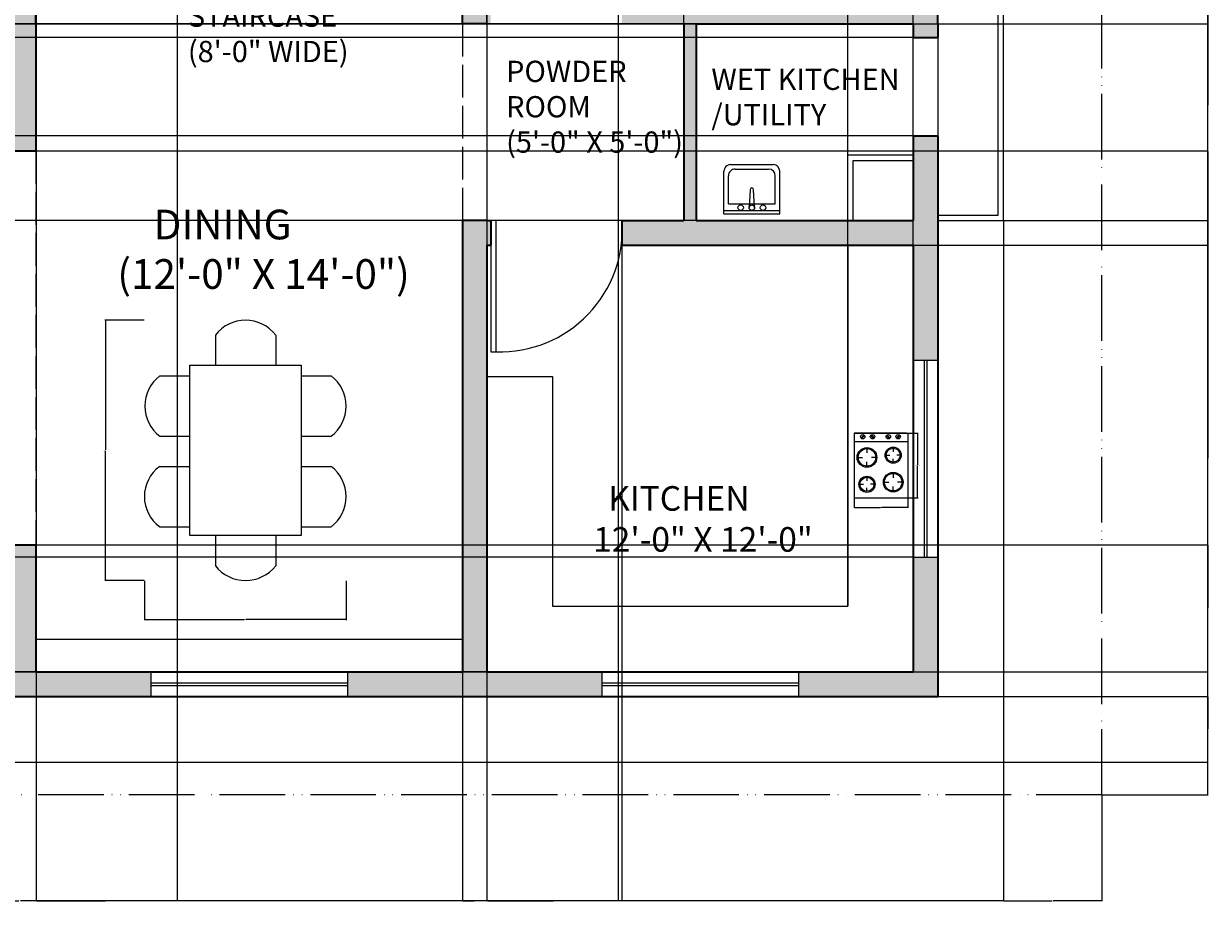
# Model space of a CAD drawing. Units: inches. Extents: x 2847 to 3693, y 1516 to 2098.
# Tile 5 of 6: x 3259 to 3693, y 1516 to 1837. Entities that reach past the tile are written whole.
import ezdxf

# ---------------------------------------------------------------- set-up
doc = ezdxf.new("R2010")
doc.units = ezdxf.units.IN
doc.linetypes.add('ACAD_ISO02W100', pattern=[15, 12, -3])
doc.linetypes.add('ACAD_ISO05W100', pattern=[33, 24, -3, 0, -3, 0, -3])
for name, color, linetype, lineweight in [('A-ANNO-DIMS', 2, 'Continuous', 18), ('A-AREA-IDEN', 7, 'Continuous', 18), ('A-DOOR', 3, 'Continuous', 18), ('A-EQPM', 9, 'Continuous', 18), ('A-FLOR', 7, 'Continuous', 25), ('A-FLOR-CASE', 8, 'Continuous', 18), ('A-FLOR-FIXT', 9, 'Continuous', 18), ('A-FLOR-OVHD', 8, 'ACAD_ISO02W100', 13), ('A-FURN', 8, 'Continuous', 18), ('A-GLAZ', 4, 'Continuous', 18), ('A-WALL', 7, 'Continuous', 35), ('C-PROP', 7, 'ACAD_ISO05W100', 18)]:
    doc.layers.add(name, color=color, linetype=linetype, lineweight=lineweight)
doc.layers.add('A-WALL-PATT', color=251, linetype='Continuous', lineweight=13, true_color=0x636466)
doc.styles.get("Standard").update_dxf_attribs({"font": 'arial.ttf'})
doc.dimstyles.get("Standard").update_dxf_attribs({"dimtxt": 0.18, "dimasz": 0.18, "dimexe": 0.18, "dimexo": 0.0625, "dimgap": 0.09, "dimtad": 0, "dimtih": 1, "dimtoh": 1, "dimdec": 4, "dimzin": 0, "dimdsep": 46, "dimtxsty": 'Standard', "dimcen": 0.09, "dimadec": 0, "dimazin": 0, "dimtfac": 1, "dimtdec": 4, "dimtofl": 0, "dimtmove": 0, "dimatfit": 3, "dimfxl": 1, "dimtolj": 1, "dimtzin": 0, "dimarcsym": 0})

# ---------------------------------------------------------------- blocks, each defined once
blk = doc.blocks.new('DINING TABLE')
for p, q in [((2443.51, 1632.65), (2443.51, 1644.65)), ((2467.51, 1632.65), (2467.51, 1644.65)), ((2479.51, 1632.65), (2479.51, 1644.65)), ((2503.51, 1632.65), (2503.51, 1644.65)), ((2427.28, 1622.52), (2439.28, 1622.52)), ((2507.03, 1622.52), (2519.03, 1622.52)), ((2427.28, 1598.52), (2439.28, 1598.52)), ((2507.03, 1598.52), (2519.03, 1598.52)), ((2443.51, 1576.39), (2443.51, 1588.39)), ((2467.51, 1576.39), (2467.51, 1588.39)), ((2479.51, 1576.39), (2479.51, 1588.39)), ((2503.51, 1576.39), (2503.51, 1588.39))]:
    blk.add_line(p, q)
blk.add_lwpolyline([(2439.28, 1632.65), (2507.03, 1632.65), (2507.03, 1588.39), (2439.28, 1588.39)], close=True)
for centre, radius, start, end in [((2455.51, 1635.3), 15.21, 37.9308, 142.0692), ((2491.51, 1635.3), 15.21, 37.9308, 142.0692), ((2436.64, 1610.52), 15.21, 127.9308, 232.0692), ((2509.67, 1610.52), 15.21, 307.9308, 52.0692), ((2455.51, 1585.74), 15.21, 217.9308, 322.0692), ((2491.51, 1585.15), 14.86, 216.1262, 323.8738)]:
    blk.add_arc(centre, radius, start, end)
blk = doc.blocks.new('A$C16A60262')
at = {"linetype": 'ByBlock'}
for p, q in [((0, 600), (0, 0)), ((488, 600), (0, 600)), ((0, 600), (500, 600)), ((0, 600), (500, 600)), ((500, 600), (500, 0)), ((500, 600), (500, 0)), ((500, 520), (0, 520)), ((119, 456), (119, 415)), ((363, 460), (363, 427)), ((38, 374), (79, 374)), ((119, 293), (119, 334)), ((201, 374), (160, 374)), ((298, 395), (331, 395)), ((363, 330), (363, 362)), ((428, 395), (396, 395)), ((363, 225), (363, 185)), ((54, 124), (87, 124)), ((119, 189), (119, 156)), ((184, 124), (152, 124)), ((282, 144), (323, 144)), ((445, 144), (404, 144)), ((0, 0), (500, 0)), ((119, 59), (119, 91)), ((363, 63), (363, 103))]:
    blk.add_line(p, q, dxfattribs=at)
for p, q in [((66, 557), (87, 579)), ((72, 552), (66, 557)), ((93, 573), (72, 552)), ((87, 579), (93, 573)), ((158, 572), (163, 578)), ((179, 551), (158, 572)), ((163, 578), (184, 557)), ((184, 557), (179, 551)), ((305, 572), (311, 578)), ((326, 551), (305, 572)), ((311, 578), (332, 557)), ((332, 557), (326, 551)), ((396, 558), (417, 580)), ((402, 553), (396, 558)), ((423, 574), (402, 553)), ((417, 580), (423, 574))]:
    blk.add_line(p, q)
for centre in [(80, 566), (171, 566), (318, 566), (409, 566)]:
    blk.add_circle(centre, 20.6)
for centre, radius in [((119, 374), 91.3), ((119, 374), 81.3), ((363, 395), 75), ((363, 395), 65), ((363, 144), 91.3), ((363, 144), 81.3), ((119, 124), 75), ((119, 124), 65)]:
    blk.add_circle(centre, radius, dxfattribs=at)
blk = doc.blocks.new('A$C5C4020F2')
for p, q in [((0.5, 0.44), (0, 0.44)), ((0, 0.44), (0, 0.06)), ((0.5, 0.44), (0.5, 0.06)), ((0.5, 0.41), (0, 0.41)), ((0.04, 0.35), (0.04, 0.1)), ((0.46, 0.35), (0.04, 0.35)), ((0.225, 0.384), (0.234, 0.224)), ((0.266, 0.224), (0.275, 0.384)), ((0.46, 0.35), (0.46, 0.1)), ((0.4, 0.04), (0.1, 0.04)), ((0.44, 0), (0.06, 0))]:
    blk.add_line(p, q)
for centre in [(0.15, 0.385), (0.25, 0.385), (0.35, 0.385)]:
    blk.add_circle(centre, 0.025)
for centre, radius, start, end in [((0.25, 0.225), 0.016, 183.2169, 356.7831), ((0.06, 0.06), 0.06, 180, 270), ((0.1, 0.1), 0.06, 180, 270), ((0.4, 0.1), 0.06, 270, 0), ((0.44, 0.06), 0.06, 270, 0)]:
    blk.add_arc(centre, radius, start, end)
blk = doc.blocks.new('WIN-GLAZ-72IN')
for p, q in [((0, 1), (72, 1)), ((0, 0), (72, 0))]:
    blk.add_line(p, q)
blk = doc.blocks.new('*D27')
at = {"layer": 'A-ANNO-DIMS', "color": 0, "lineweight": -2, "transparency": 16777216}
for p, q in [((3303.45, 1728.67), (3289.06, 1728.67)), ((3289.24, 1728.49), (3289.24, 1681.27)), ((3289.24, 1633.69), (3289.24, 1680.91)), ((3303.45, 1633.51), (3289.06, 1633.51))]:
    blk.add_line(p, q, dxfattribs=at)
at = {"layer": 'A-ANNO-DIMS', "color": 0, "transparency": 16777216}
for points in [[(3289.21, 1728.49), (3289.27, 1728.49), (3289.24, 1728.67)], [(3289.21, 1633.69), (3289.27, 1633.69), (3289.24, 1633.51)]]:
    blk.add_solid(points, dxfattribs=at)
at = {"layer": 'Defpoints', "color": 0, "transparency": 16777216}
for p in [(3303.51, 1728.67), (3289.24, 1633.51), (3303.51, 1633.51)]:
    blk.add_point(p, dxfattribs=at)
at = {"layer": 'A-ANNO-DIMS', "color": 0, "transparency": 16777216, "insert": (3289.24, 1681.09), "char_height": 0.18, "attachment_point": 5}
blk.add_mtext('\\A1;DINING SET 95', dxfattribs=at)
blk = doc.blocks.new('*D28')
at = {"layer": 'A-ANNO-DIMS', "color": 0, "lineweight": -2, "transparency": 16777216}
for p, q in [((3303.51, 1633.45), (3303.51, 1619.05)), ((3377.29, 1633.45), (3377.29, 1619.05)), ((3303.69, 1619.23), (3340.18, 1619.23)), ((3377.11, 1619.23), (3340.62, 1619.23))]:
    blk.add_line(p, q, dxfattribs=at)
at = {"layer": 'A-ANNO-DIMS', "color": 0, "transparency": 16777216}
for points in [[(3303.69, 1619.26), (3303.69, 1619.2), (3303.51, 1619.23)], [(3377.11, 1619.26), (3377.11, 1619.2), (3377.29, 1619.23)]]:
    blk.add_solid(points, dxfattribs=at)
at = {"layer": 'Defpoints', "color": 0, "transparency": 16777216}
for p in [(3303.51, 1633.51), (3377.29, 1633.51), (3377.29, 1619.23)]:
    blk.add_point(p, dxfattribs=at)
at = {"layer": 'A-ANNO-DIMS', "color": 0, "transparency": 16777216, "insert": (3340.4, 1619.23), "char_height": 0.18, "attachment_point": 5}
blk.add_mtext('\\A1;74', dxfattribs=at)
blk = doc.blocks.new('*D29')
at = {"layer": 'A-ANNO-DIMS', "color": 0, "lineweight": -2, "transparency": 16777216}
for p, q in [((3582.95, 1687.44), (3586.61, 1687.44)), ((3586.43, 1687.26), (3586.43, 1675.81)), ((3586.43, 1663.99), (3586.43, 1675.44)), ((3582.95, 1663.81), (3586.61, 1663.81))]:
    blk.add_line(p, q, dxfattribs=at)
at = {"layer": 'A-ANNO-DIMS', "color": 0, "transparency": 16777216}
for points in [[(3586.4, 1687.26), (3586.46, 1687.26), (3586.43, 1687.44)], [(3586.4, 1663.99), (3586.46, 1663.99), (3586.43, 1663.81)]]:
    blk.add_solid(points, dxfattribs=at)
at = {"layer": 'Defpoints', "color": 0, "transparency": 16777216}
for p in [(3582.89, 1687.44), (3586.43, 1687.44), (3582.89, 1663.81)]:
    blk.add_point(p, dxfattribs=at)
at = {"layer": 'A-ANNO-DIMS', "color": 0, "transparency": 16777216, "insert": (3586.43, 1675.63), "char_height": 0.18, "attachment_point": 5}
blk.add_mtext('\\A1;COOKTOP 24', dxfattribs=at)
blk = doc.blocks.new('*D30')
at = {"layer": 'A-ANNO-DIMS', "color": 0, "lineweight": -2, "transparency": 16777216}
for p, q in [((3563.2, 1663.75), (3563.2, 1660.09)), ((3563.38, 1660.27), (3572.82, 1660.27)), ((3582.71, 1660.27), (3573.26, 1660.27)), ((3582.89, 1663.75), (3582.89, 1660.09))]:
    blk.add_line(p, q, dxfattribs=at)
at = {"layer": 'A-ANNO-DIMS', "color": 0, "transparency": 16777216}
for points in [[(3563.38, 1660.3), (3563.38, 1660.24), (3563.2, 1660.27)], [(3582.71, 1660.3), (3582.71, 1660.24), (3582.89, 1660.27)]]:
    blk.add_solid(points, dxfattribs=at)
at = {"layer": 'Defpoints', "color": 0, "transparency": 16777216}
for p in [(3563.2, 1663.81), (3582.89, 1663.81), (3582.89, 1660.27)]:
    blk.add_point(p, dxfattribs=at)
at = {"layer": 'A-ANNO-DIMS', "color": 0, "transparency": 16777216, "insert": (3573.04, 1660.27), "char_height": 0.18, "attachment_point": 5}
blk.add_mtext('\\A1;20', dxfattribs=at)
blk = doc.blocks.new('*D36')
at = {"layer": 'A-ANNO-DIMS', "color": 0, "lineweight": -2, "transparency": 16777216}
for p, q in [((3653.91, 2059.12), (3692.73, 2059.12)), ((3692.55, 2058.94), (3692.55, 1807.3)), ((3692.55, 1555.3), (3692.55, 1806.94)), ((3653.91, 1555.12), (3692.73, 1555.12))]:
    blk.add_line(p, q, dxfattribs=at)
at = {"layer": 'A-ANNO-DIMS', "color": 0, "transparency": 16777216}
for points in [[(3692.52, 2058.94), (3692.58, 2058.94), (3692.55, 2059.12)], [(3692.52, 1555.3), (3692.58, 1555.3), (3692.55, 1555.12)]]:
    blk.add_solid(points, dxfattribs=at)
at = {"layer": 'Defpoints', "color": 0, "transparency": 16777216}
for p in [(3653.85, 2059.12), (3692.55, 2059.12), (3653.85, 1555.12)]:
    blk.add_point(p, dxfattribs=at)
at = {"layer": 'A-ANNO-DIMS', "color": 0, "transparency": 16777216, "insert": (3692.55, 1807.12), "char_height": 0.18, "attachment_point": 5}
blk.add_mtext('\\A1;504', dxfattribs=at)
blk = doc.blocks.new('*D37')
at = {"layer": 'A-ANNO-DIMS', "color": 0, "lineweight": -2, "transparency": 16777216}
for p, q in [((3617.85, 1765.06), (3617.85, 1516.24)), ((2897.85, 1591.06), (2897.85, 1516.24)), ((2898.03, 1516.42), (3257.56, 1516.42)), ((3617.67, 1516.42), (3258.13, 1516.42))]:
    blk.add_line(p, q, dxfattribs=at)
at = {"layer": 'A-ANNO-DIMS', "color": 0, "transparency": 16777216}
for points in [[(2898.03, 1516.45), (2898.03, 1516.39), (2897.85, 1516.42)], [(3617.67, 1516.45), (3617.67, 1516.39), (3617.85, 1516.42)]]:
    blk.add_solid(points, dxfattribs=at)
at = {"layer": 'Defpoints', "color": 0, "transparency": 16777216}
for p in [(3617.85, 1765.12), (2897.85, 1591.12), (3617.85, 1516.42)]:
    blk.add_point(p, dxfattribs=at)
at = {"layer": 'A-ANNO-DIMS', "color": 0, "transparency": 16777216, "insert": (3257.85, 1516.42), "char_height": 0.18, "attachment_point": 5}
blk.add_mtext('\\A1;720', dxfattribs=at)
blk = doc.blocks.new('*D46')
at = {"layer": 'A-ANNO-DIMS', "color": 0, "lineweight": -2, "transparency": 16777216}
for p, q in [((3584.91, 1756.12), (3692.73, 1756.12)), ((3692.55, 1755.94), (3692.55, 1678.3)), ((3692.55, 1600.3), (3692.55, 1677.94)), ((3584.91, 1600.12), (3692.73, 1600.12))]:
    blk.add_line(p, q, dxfattribs=at)
at = {"layer": 'A-ANNO-DIMS', "color": 0, "transparency": 16777216}
for points in [[(3692.52, 1755.94), (3692.58, 1755.94), (3692.55, 1756.12)], [(3692.52, 1600.3), (3692.58, 1600.3), (3692.55, 1600.12)]]:
    blk.add_solid(points, dxfattribs=at)
at = {"layer": 'Defpoints', "color": 0, "transparency": 16777216}
for p in [(3584.85, 1756.12), (3692.55, 1756.12), (3584.85, 1600.12)]:
    blk.add_point(p, dxfattribs=at)
at = {"layer": 'A-ANNO-DIMS', "color": 0, "transparency": 16777216, "insert": (3692.55, 1678.12), "char_height": 0.18, "attachment_point": 5}
blk.add_mtext('\\A1;156', dxfattribs=at)
blk = doc.blocks.new('*D47')
at = {"layer": 'A-ANNO-DIMS', "color": 0, "lineweight": -2, "transparency": 16777216}
for p, q in [((3617.91, 1960.12), (3692.73, 1960.12)), ((3692.55, 1959.94), (3692.55, 1862.8)), ((3692.55, 1765.3), (3692.55, 1862.44)), ((3617.91, 1765.12), (3692.73, 1765.12))]:
    blk.add_line(p, q, dxfattribs=at)
at = {"layer": 'A-ANNO-DIMS', "color": 0, "transparency": 16777216}
for points in [[(3692.52, 1959.94), (3692.58, 1959.94), (3692.55, 1960.12)], [(3692.52, 1765.3), (3692.58, 1765.3), (3692.55, 1765.12)]]:
    blk.add_solid(points, dxfattribs=at)
at = {"layer": 'Defpoints', "color": 0, "transparency": 16777216}
for p in [(3617.85, 1960.12), (3692.55, 1960.12), (3617.85, 1765.12)]:
    blk.add_point(p, dxfattribs=at)
at = {"layer": 'A-ANNO-DIMS', "color": 0, "transparency": 16777216, "insert": (3692.55, 1862.62), "char_height": 0.18, "attachment_point": 5}
blk.add_mtext('\\A1;195', dxfattribs=at)
blk = doc.blocks.new('*D50')
at = {"layer": 'A-ANNO-DIMS', "color": 0, "lineweight": -2, "transparency": 16777216}
for p, q in [((2989.41, 2011.12), (3692.73, 2011.12)), ((3692.55, 2010.94), (3692.55, 1924.3)), ((3692.55, 1837.3), (3692.55, 1923.94)), ((2989.41, 1837.12), (3692.73, 1837.12))]:
    blk.add_line(p, q, dxfattribs=at)
at = {"layer": 'A-ANNO-DIMS', "color": 0, "transparency": 16777216}
for points in [[(3692.52, 2010.94), (3692.58, 2010.94), (3692.55, 2011.12)], [(3692.52, 1837.3), (3692.58, 1837.3), (3692.55, 1837.12)]]:
    blk.add_solid(points, dxfattribs=at)
at = {"layer": 'Defpoints', "color": 0, "transparency": 16777216}
for p in [(2989.35, 2011.12), (3692.55, 2011.12), (2989.35, 1837.12)]:
    blk.add_point(p, dxfattribs=at)
at = {"layer": 'A-ANNO-DIMS', "color": 0, "transparency": 16777216, "insert": (3692.55, 1924.12), "char_height": 0.18, "attachment_point": 5}
blk.add_mtext('\\A1;174', dxfattribs=at)
blk = doc.blocks.new('*D52')
at = {"layer": 'A-ANNO-DIMS', "color": 0, "lineweight": -2, "transparency": 16777216}
for p, q in [((3505.28, 1837.12), (2846.97, 1837.12)), ((2847.15, 1836.94), (2847.15, 1801.3)), ((2847.15, 1765.3), (2847.15, 1800.94)), ((3505.28, 1765.12), (2846.97, 1765.12))]:
    blk.add_line(p, q, dxfattribs=at)
at = {"layer": 'A-ANNO-DIMS', "color": 0, "transparency": 16777216}
for points in [[(2847.12, 1836.94), (2847.18, 1836.94), (2847.15, 1837.12)], [(2847.12, 1765.3), (2847.18, 1765.3), (2847.15, 1765.12)]]:
    blk.add_solid(points, dxfattribs=at)
at = {"layer": 'Defpoints', "color": 0, "transparency": 16777216}
for p in [(2847.15, 1837.12), (3505.35, 1837.12), (3505.35, 1765.12)]:
    blk.add_point(p, dxfattribs=at)
at = {"layer": 'A-ANNO-DIMS', "color": 0, "transparency": 16777216, "insert": (2847.15, 1801.12), "char_height": 0.18, "attachment_point": 5}
blk.add_mtext('\\A1;72', dxfattribs=at)
blk = doc.blocks.new('*D53')
at = {"layer": 'A-ANNO-DIMS', "color": 0, "lineweight": -2, "transparency": 16777216}
for p, q in [((3428.85, 1837.18), (3428.85, 2098)), ((3500.85, 1837.18), (3500.85, 2098)), ((3429.03, 2097.82), (3464.63, 2097.82)), ((3500.67, 2097.82), (3465.06, 2097.82))]:
    blk.add_line(p, q, dxfattribs=at)
at = {"layer": 'A-ANNO-DIMS', "color": 0, "transparency": 16777216}
for points in [[(3429.03, 2097.85), (3429.03, 2097.79), (3428.85, 2097.82)], [(3500.67, 2097.85), (3500.67, 2097.79), (3500.85, 2097.82)]]:
    blk.add_solid(points, dxfattribs=at)
at = {"layer": 'Defpoints', "color": 0, "transparency": 16777216}
for p in [(3500.85, 2097.82), (3428.85, 1837.12), (3500.85, 1837.12)]:
    blk.add_point(p, dxfattribs=at)
at = {"layer": 'A-ANNO-DIMS', "color": 0, "transparency": 16777216, "insert": (3464.85, 2097.82), "char_height": 0.18, "attachment_point": 5}
blk.add_mtext('\\A1;72', dxfattribs=at)
blk = doc.blocks.new('*D57')
at = {"layer": 'A-ANNO-DIMS', "color": 0, "lineweight": -2, "transparency": 16777216}
for p, q in [((3263.85, 1854.46), (3263.85, 1516.24)), ((3315.45, 1854.46), (3315.45, 1516.24)), ((3264.03, 1516.42), (3289.32, 1516.42)), ((3315.27, 1516.42), (3289.97, 1516.42))]:
    blk.add_line(p, q, dxfattribs=at)
at = {"layer": 'A-ANNO-DIMS', "color": 0, "transparency": 16777216}
for points in [[(3264.03, 1516.45), (3264.03, 1516.39), (3263.85, 1516.42)], [(3315.27, 1516.45), (3315.27, 1516.39), (3315.45, 1516.42)]]:
    blk.add_solid(points, dxfattribs=at)
at = {"layer": 'Defpoints', "color": 0, "transparency": 16777216}
for p in [(3263.85, 1854.52), (3315.45, 1854.52), (3315.45, 1516.42)]:
    blk.add_point(p, dxfattribs=at)
at = {"layer": 'A-ANNO-DIMS', "color": 0, "transparency": 16777216, "insert": (3289.65, 1516.42), "char_height": 0.18, "attachment_point": 5}
blk.add_mtext('\\A1;51.6', dxfattribs=at)
blk = doc.blocks.new('*D60')
at = {"layer": 'A-ANNO-DIMS', "color": 0, "lineweight": -2, "transparency": 16777216}
for p, q in [((3428.85, 1765.06), (3428.85, 1516.24)), ((3478.26, 1765.06), (3478.26, 1516.24)), ((3429.03, 1516.42), (3453.17, 1516.42)), ((3478.08, 1516.42), (3453.93, 1516.42))]:
    blk.add_line(p, q, dxfattribs=at)
at = {"layer": 'A-ANNO-DIMS', "color": 0, "transparency": 16777216}
for points in [[(3429.03, 1516.45), (3429.03, 1516.39), (3428.85, 1516.42)], [(3478.08, 1516.45), (3478.08, 1516.39), (3478.26, 1516.42)]]:
    blk.add_solid(points, dxfattribs=at)
at = {"layer": 'Defpoints', "color": 0, "transparency": 16777216}
for p in [(3428.85, 1765.12), (3478.26, 1765.12), (3478.26, 1516.42)]:
    blk.add_point(p, dxfattribs=at)
at = {"layer": 'A-ANNO-DIMS', "color": 0, "transparency": 16777216, "insert": (3453.55, 1516.42), "char_height": 0.18, "attachment_point": 5}
blk.add_mtext('\\A1;49.41', dxfattribs=at)
blk = doc.blocks.new('*D62')
at = {"layer": 'A-ANNO-DIMS', "color": 0, "lineweight": -2, "transparency": 16777216}
for p, q in [((3617.85, 1765.06), (3617.85, 1516.24)), ((3653.85, 1555.06), (3653.85, 1516.24)), ((3618.03, 1516.42), (3635.63, 1516.42)), ((3653.67, 1516.42), (3636.06, 1516.42))]:
    blk.add_line(p, q, dxfattribs=at)
at = {"layer": 'A-ANNO-DIMS', "color": 0, "transparency": 16777216}
for points in [[(3618.03, 1516.45), (3618.03, 1516.39), (3617.85, 1516.42)], [(3653.67, 1516.45), (3653.67, 1516.39), (3653.85, 1516.42)]]:
    blk.add_solid(points, dxfattribs=at)
at = {"layer": 'Defpoints', "color": 0, "transparency": 16777216}
for p in [(3617.85, 1765.12), (3653.85, 1555.12), (3653.85, 1516.42)]:
    blk.add_point(p, dxfattribs=at)
at = {"layer": 'A-ANNO-DIMS', "color": 0, "transparency": 16777216, "insert": (3635.85, 1516.42), "char_height": 0.18, "attachment_point": 5}
blk.add_mtext('\\A1;36', dxfattribs=at)
blk = doc.blocks.new('*D64')
at = {"layer": 'A-ANNO-DIMS', "color": 0, "lineweight": -2, "transparency": 16777216}
for p, q in [((2921.91, 1591.12), (3692.73, 1591.12)), ((3692.55, 1590.94), (3692.55, 1579.3)), ((3692.55, 1567.3), (3692.55, 1578.94)), ((2921.91, 1567.12), (3692.73, 1567.12))]:
    blk.add_line(p, q, dxfattribs=at)
at = {"layer": 'A-ANNO-DIMS', "color": 0, "transparency": 16777216}
for points in [[(3692.52, 1590.94), (3692.58, 1590.94), (3692.55, 1591.12)], [(3692.52, 1567.3), (3692.58, 1567.3), (3692.55, 1567.12)]]:
    blk.add_solid(points, dxfattribs=at)
at = {"layer": 'Defpoints', "color": 0, "transparency": 16777216}
for p in [(2921.85, 1591.12), (3692.55, 1591.12), (2921.85, 1567.12)]:
    blk.add_point(p, dxfattribs=at)
at = {"layer": 'A-ANNO-DIMS', "color": 0, "transparency": 16777216, "insert": (3692.55, 1579.12), "char_height": 0.18, "attachment_point": 5}
blk.add_mtext('\\A1;24', dxfattribs=at)
blk = doc.blocks.new('*D67')
at = {"layer": 'A-ANNO-DIMS', "color": 0, "lineweight": -2, "transparency": 16777216}
for p, q in [((3428.85, 2002.06), (3428.85, 1516.24)), ((3476.85, 2002.06), (3476.85, 1516.24)), ((3429.03, 1516.42), (3452.62, 1516.42)), ((3476.67, 1516.42), (3453.07, 1516.42))]:
    blk.add_line(p, q, dxfattribs=at)
at = {"layer": 'A-ANNO-DIMS', "color": 0, "transparency": 16777216}
for points in [[(3429.03, 1516.45), (3429.03, 1516.39), (3428.85, 1516.42)], [(3476.67, 1516.45), (3476.67, 1516.39), (3476.85, 1516.42)]]:
    blk.add_solid(points, dxfattribs=at)
at = {"layer": 'Defpoints', "color": 0, "transparency": 16777216}
for p in [(3428.85, 2002.12), (3476.85, 2002.12), (3476.85, 1516.42)]:
    blk.add_point(p, dxfattribs=at)
at = {"layer": 'A-ANNO-DIMS', "color": 0, "transparency": 16777216, "insert": (3452.85, 1516.42), "char_height": 0.18, "attachment_point": 5}
blk.add_mtext('\\A1;48', dxfattribs=at)
blk = doc.blocks.new('*D68')
at = {"layer": 'A-ANNO-DIMS', "color": 0, "lineweight": -2, "transparency": 16777216}
for p, q in [((3560.85, 1624.18), (3560.85, 2098)), ((3584.85, 1600.18), (3584.85, 2098)), ((3561.03, 2097.82), (3572.63, 2097.82)), ((3584.67, 2097.82), (3573.07, 2097.82))]:
    blk.add_line(p, q, dxfattribs=at)
at = {"layer": 'A-ANNO-DIMS', "color": 0, "transparency": 16777216}
for points in [[(3561.03, 2097.85), (3561.03, 2097.79), (3560.85, 2097.82)], [(3584.67, 2097.85), (3584.67, 2097.79), (3584.85, 2097.82)]]:
    blk.add_solid(points, dxfattribs=at)
at = {"layer": 'Defpoints', "color": 0, "transparency": 16777216}
for p in [(3560.85, 2097.82), (3560.85, 1624.12), (3584.85, 1600.12)]:
    blk.add_point(p, dxfattribs=at)
at = {"layer": 'A-ANNO-DIMS', "color": 0, "transparency": 16777216, "insert": (3572.85, 2097.82), "char_height": 0.18, "attachment_point": 5}
blk.add_mtext('\\A1;24', dxfattribs=at)
blk = doc.blocks.new('*D70')
at = {"layer": 'A-ANNO-DIMS', "color": 0, "lineweight": -2, "transparency": 16777216}
for p, q in [((3419.85, 1600.06), (3419.85, 1516.24)), ((3428.85, 1600.06), (3428.85, 1516.24)), ((3420.03, 1516.42), (3424.2, 1516.42)), ((3428.67, 1516.42), (3424.49, 1516.42))]:
    blk.add_line(p, q, dxfattribs=at)
at = {"layer": 'A-ANNO-DIMS', "color": 0, "transparency": 16777216}
for points in [[(3420.03, 1516.45), (3420.03, 1516.39), (3419.85, 1516.42)], [(3428.67, 1516.45), (3428.67, 1516.39), (3428.85, 1516.42)]]:
    blk.add_solid(points, dxfattribs=at)
at = {"layer": 'Defpoints', "color": 0, "transparency": 16777216}
for p in [(3419.85, 1600.12), (3428.85, 1600.12), (3419.85, 1516.42)]:
    blk.add_point(p, dxfattribs=at)
at = {"layer": 'A-ANNO-DIMS', "color": 0, "transparency": 16777216, "insert": (3424.35, 1516.42), "char_height": 0.18, "attachment_point": 5}
blk.add_mtext('\\A1;9', dxfattribs=at)
blk = doc.blocks.new('*D71')
at = {"layer": 'A-ANNO-DIMS', "color": 0, "lineweight": -2, "transparency": 16777216}
for p, q in [((3254.91, 1790.62), (3692.73, 1790.62)), ((3692.55, 1790.44), (3692.55, 1718.8)), ((3692.55, 1646.8), (3692.55, 1718.44)), ((3254.91, 1646.62), (3692.73, 1646.62))]:
    blk.add_line(p, q, dxfattribs=at)
at = {"layer": 'A-ANNO-DIMS', "color": 0, "transparency": 16777216}
for points in [[(3692.52, 1790.44), (3692.58, 1790.44), (3692.55, 1790.62)], [(3692.52, 1646.8), (3692.58, 1646.8), (3692.55, 1646.62)]]:
    blk.add_solid(points, dxfattribs=at)
at = {"layer": 'Defpoints', "color": 0, "transparency": 16777216}
for p in [(3254.85, 1790.62), (3692.55, 1790.62), (3254.85, 1646.62)]:
    blk.add_point(p, dxfattribs=at)
at = {"layer": 'A-ANNO-DIMS', "color": 0, "transparency": 16777216, "insert": (3692.55, 1718.62), "char_height": 0.18, "attachment_point": 5}
blk.add_mtext('\\A1;144', dxfattribs=at)
blk = doc.blocks.new('*D72')
at = {"layer": 'A-ANNO-DIMS', "color": 0, "lineweight": -2, "transparency": 16777216}
for p, q in [((3254.91, 1646.62), (3692.73, 1646.62)), ((3692.55, 1646.44), (3692.55, 1623.55)), ((3692.55, 1600.3), (3692.55, 1623.19)), ((3254.91, 1600.12), (3692.73, 1600.12))]:
    blk.add_line(p, q, dxfattribs=at)
at = {"layer": 'A-ANNO-DIMS', "color": 0, "transparency": 16777216}
for points in [[(3692.52, 1646.44), (3692.58, 1646.44), (3692.55, 1646.62)], [(3692.52, 1600.3), (3692.58, 1600.3), (3692.55, 1600.12)]]:
    blk.add_solid(points, dxfattribs=at)
at = {"layer": 'Defpoints', "color": 0, "transparency": 16777216}
for p in [(3254.85, 1646.62), (3692.55, 1646.62), (3254.85, 1600.12)]:
    blk.add_point(p, dxfattribs=at)
at = {"layer": 'A-ANNO-DIMS', "color": 0, "transparency": 16777216, "insert": (3692.55, 1623.37), "char_height": 0.18, "attachment_point": 5}
blk.add_mtext('\\A1;46.5', dxfattribs=at)
blk = doc.blocks.new('*D76')
at = {"layer": 'A-ANNO-DIMS', "color": 0, "lineweight": -2, "transparency": 16777216}
for p, q in [((3584.78, 1642.12), (2846.97, 1642.12)), ((2847.15, 1641.94), (2847.15, 1621.3)), ((2847.15, 1600.3), (2847.15, 1620.94)), ((3584.78, 1600.12), (2846.97, 1600.12))]:
    blk.add_line(p, q, dxfattribs=at)
at = {"layer": 'A-ANNO-DIMS', "color": 0, "transparency": 16777216}
for points in [[(2847.12, 1641.94), (2847.18, 1641.94), (2847.15, 1642.12)], [(2847.12, 1600.3), (2847.18, 1600.3), (2847.15, 1600.12)]]:
    blk.add_solid(points, dxfattribs=at)
at = {"layer": 'Defpoints', "color": 0, "transparency": 16777216}
for p in [(2847.15, 1642.12), (3584.85, 1642.12), (3584.85, 1600.12)]:
    blk.add_point(p, dxfattribs=at)
at = {"layer": 'A-ANNO-DIMS', "color": 0, "transparency": 16777216, "insert": (2847.15, 1621.12), "char_height": 0.18, "attachment_point": 5}
blk.add_mtext('\\A1;42', dxfattribs=at)
blk = doc.blocks.new('*D77')
at = {"layer": 'A-ANNO-DIMS', "color": 0, "lineweight": -2, "transparency": 16777216}
for p, q in [((3584.78, 1832.08), (2846.97, 1832.08)), ((2847.15, 1831.9), (2847.15, 1814.27)), ((2847.15, 1796.26), (2847.15, 1813.9)), ((3584.78, 1796.08), (2846.97, 1796.08))]:
    blk.add_line(p, q, dxfattribs=at)
at = {"layer": 'A-ANNO-DIMS', "color": 0, "transparency": 16777216}
for points in [[(2847.12, 1831.9), (2847.18, 1831.9), (2847.15, 1832.08)], [(2847.12, 1796.26), (2847.18, 1796.26), (2847.15, 1796.08)]]:
    blk.add_solid(points, dxfattribs=at)
at = {"layer": 'Defpoints', "color": 0, "transparency": 16777216}
for p in [(2847.15, 1832.08), (3584.85, 1832.08), (3584.85, 1796.08)]:
    blk.add_point(p, dxfattribs=at)
at = {"layer": 'A-ANNO-DIMS', "color": 0, "transparency": 16777216, "insert": (2847.15, 1814.08), "char_height": 0.18, "attachment_point": 5}
blk.add_mtext('\\A1;36', dxfattribs=at)
blk = doc.blocks.new('*D78')
at = {"layer": 'A-ANNO-DIMS', "color": 0, "lineweight": -2, "transparency": 16777216}
for p, q in [((3584.78, 1796.08), (2846.97, 1796.08)), ((2847.15, 1795.9), (2847.15, 1780.78)), ((2847.15, 1765.3), (2847.15, 1780.42)), ((3584.78, 1765.12), (2846.97, 1765.12))]:
    blk.add_line(p, q, dxfattribs=at)
at = {"layer": 'A-ANNO-DIMS', "color": 0, "transparency": 16777216}
for points in [[(2847.12, 1795.9), (2847.18, 1795.9), (2847.15, 1796.08)], [(2847.12, 1765.3), (2847.18, 1765.3), (2847.15, 1765.12)]]:
    blk.add_solid(points, dxfattribs=at)
at = {"layer": 'Defpoints', "color": 0, "transparency": 16777216}
for p in [(2847.15, 1796.08), (3584.85, 1796.08), (3584.85, 1765.12)]:
    blk.add_point(p, dxfattribs=at)
at = {"layer": 'A-ANNO-DIMS', "color": 0, "transparency": 16777216, "insert": (2847.15, 1780.6), "char_height": 0.18, "attachment_point": 5}
blk.add_mtext('\\A1;30.965', dxfattribs=at)

msp = doc.modelspace()

# ---------------------------------------------------------------- hatches: boundary and pattern name
at = {"layer": 'A-WALL-PATT'}
h = msp.add_hatch(color=256, dxfattribs=at)
h.dxf.hatch_style = 1
h.paths.add_polyline_path([(2998.3457, 2002.118), (3178.3457, 2002.118), (3178.3457, 1944.368, -0.0341147), (3182.8457, 1944.4698), (3182.8457, 2002.118), (3200.8457, 2002.118), (3200.8457, 2011.118), (2989.3457, 2011.118), (2989.3457, 1960.118), (2998.3457, 1960.118)])
h.paths.add_polyline_path([(2998.3457, 1888.118), (2989.3457, 1888.118), (2989.3457, 1837.118), (3089.8457, 1837.118), (3089.8457, 1778.618), (3098.8457, 1778.618), (3098.8457, 1837.118), (3130.3457, 1837.118, -0.05293254), (3130.1282, 1846.118), (2998.3457, 1846.118)])
h.paths.add_polyline_path([(3263.8457, 2002.118), (3311.8457, 2002.118), (3311.8457, 2011.118), (3263.8457, 2011.118), (3236.8457, 2011.118), (3236.8457, 2002.118), (3254.8457, 2002.118), (3254.8457, 1908.368), (3182.8457, 1908.368), (3178.3457, 1908.368), (3178.3457, 1886.993), (3182.8457, 1886.993), (3182.8457, 1903.868), (3254.8457, 1903.868), (3254.8457, 1846.118), (3182.8457, 1846.118), (3182.8457, 1850.993), (3178.3457, 1850.993), (3178.3457, 1837.118), (3254.8457, 1837.118), (3254.8457, 1790.618), (3263.8457, 1790.618), (3263.8457, 1837.118)])
h.paths.add_polyline_path([(2930.8457, 1837.118), (2921.8457, 1837.118), (2921.8457, 1828.118), (2930.8457, 1828.118)])
h.paths.add_polyline_path([(2930.8457, 1600.118), (2921.8457, 1600.118), (2921.8457, 1591.118), (2930.8457, 1591.118)])
h.paths.add_polyline_path([(3098.8457, 1658.618), (3089.8457, 1658.618), (3089.8457, 1591.118), (3140.8457, 1591.118), (3140.8457, 1600.118), (3098.8457, 1600.118)])
h.paths.add_polyline_path([(3305.8457, 1600.118), (3263.8457, 1600.118), (3263.8457, 1646.618), (3254.8457, 1646.618), (3254.8457, 1600.118), (3212.8457, 1600.118), (3212.8457, 1591.118), (3254.8457, 1591.118), (3305.8457, 1591.118)])
h.paths.add_polyline_path([(3470.8457, 1600.118), (3428.8457, 1600.118), (3428.8457, 1756.118), (3430.26, 1756.118), (3430.26, 1765.118), (3428.8457, 1765.118), (3419.8457, 1765.118), (3419.8457, 1600.118), (3377.8457, 1600.118), (3377.8457, 1591.118), (3470.8457, 1591.118)])
h.paths.add_polyline_path([(3593.8457, 1642.118), (3584.8457, 1642.118), (3584.8457, 1600.118), (3542.8457, 1600.118), (3542.8457, 1591.118), (3593.8457, 1591.118)])
h.paths.add_polyline_path([(3593.8457, 1796.083), (3584.8457, 1796.083), (3584.8457, 1765.118), (3505.3457, 1765.118), (3505.3457, 1837.118), (3584.8457, 1837.118), (3584.8457, 1832.083), (3593.8457, 1832.083), (3593.8457, 1837.118), (3593.8457, 1924.118), (3584.8457, 1924.118), (3584.8457, 1846.118), (3478.26, 1846.118), (3478.26, 1837.118), (3500.8457, 1837.118), (3500.8457, 1765.118), (3478.26, 1765.118, -0.03536449), (3478.26, 1758.7816), (3478.26, 1756.118), (3584.8457, 1756.118), (3584.8457, 1714.118), (3593.8457, 1714.118)])
h.paths.add_polyline_path([(3593.8457, 2011.118), (3536.8457, 2011.118), (3536.8457, 2002.118), (3584.8457, 2002.118), (3584.8457, 1960.118), (3593.8457, 1960.118)])
h.paths.add_polyline_path([(3476.8457, 2011.118), (3371.8457, 2011.118), (3371.8457, 2002.118), (3419.8457, 2002.118), (3419.8457, 1837.118), (3428.8457, 1837.118), (3430.26, 1837.118), (3430.26, 1846.118), (3428.8457, 1846.118), (3428.8457, 2002.118), (3476.8457, 2002.118)])

# ---------------------------------------------------------------- linework, layer by layer
at = {"layer": 'A-DOOR'}
for p, q in [((3430.26, 1765.118), (3430.26, 1717.118)), ((3432.26, 1765.118), (3430.26, 1765.118)), ((3432.26, 1717.118), (3432.26, 1765.118)), ((3430.26, 1717.118), (3432.26, 1717.118))]:
    msp.add_line(p, q, dxfattribs=at)
msp.add_arc((3433.5224, 1761.9498), 44.8496, 268.386967, 4.050783, dxfattribs=at)
at = {"layer": 'A-FLOR'}
for p, q in [((3617.8457, 1765.118), (3617.8457, 1960.118)), ((3615.8457, 1767.118), (3615.8457, 1958.118)), ((3593.8457, 1832.083), (3593.8457, 1796.083)), ((3593.8457, 1767.118), (3615.8457, 1767.118)), ((3593.8457, 1765.118), (3617.8457, 1765.118))]:
    msp.add_line(p, q, dxfattribs=at)
at = {"layer": 'A-FLOR-CASE'}
for p, q in [((3560.8457, 1765.118), (3560.8457, 1789.118)), ((3560.8457, 1789.118), (3584.8457, 1789.118)), ((3562.8457, 1765.118), (3562.8457, 1787.118)), ((3562.8457, 1787.118), (3584.8457, 1787.118)), ((3560.8457, 1756.118), (3560.8457, 1624.118)), ((3428.8457, 1708.118), (3452.8457, 1708.118)), ((3452.8457, 1708.118), (3452.8457, 1624.118)), ((3452.8457, 1624.118), (3560.8457, 1624.118)), ((3263.8457, 1612.118), (3419.8457, 1612.118))]:
    msp.add_line(p, q, dxfattribs=at)
at = {"layer": 'A-FLOR-OVHD'}
for p, q in [((3419.8457, 1837.118), (3419.8457, 1765.118)), ((3428.8457, 1837.118), (3428.8457, 1765.118)), ((3263.8457, 1790.618), (3263.8457, 1646.618))]:
    msp.add_line(p, q, dxfattribs=at)
at = {"layer": 'A-GLAZ'}
for p, q in [((3584.8457, 1714.118), (3593.8457, 1714.118)), ((3584.8457, 1642.118), (3593.8457, 1642.118)), ((3305.8457, 1600.118), (3305.8457, 1591.118)), ((3377.8457, 1600.118), (3377.8457, 1591.118)), ((3470.8457, 1600.118), (3470.8457, 1591.118)), ((3542.8457, 1600.118), (3542.8457, 1591.118))]:
    msp.add_line(p, q, dxfattribs=at)
at = {"layer": 'A-WALL'}
for p, q in [((3593.8457, 1837.118), (3593.8457, 2011.118)), ((3263.8457, 1837.118), (3263.8457, 2002.118)), ((3419.8457, 1837.118), (3419.8457, 2002.118)), ((3263.8457, 1837.118), (3263.8457, 1790.618)), ((3428.8457, 1837.118), (3419.8457, 1837.118)), ((3500.8457, 1837.118), (3500.8457, 1765.118)), ((3505.3457, 1837.118), (3505.3457, 1765.118)), ((3505.3457, 1837.118), (3584.8457, 1837.118)), ((3584.8457, 1837.118), (3584.8457, 1832.083)), ((3593.8457, 1837.118), (3593.8457, 1832.083)), ((3584.8457, 1832.083), (3593.8457, 1832.083)), ((3584.8457, 1796.083), (3593.8457, 1796.083)), ((3584.8457, 1796.083), (3584.8457, 1765.118)), ((3593.8457, 1796.083), (3593.8457, 1591.118)), ((3254.8457, 1790.618), (3263.8457, 1790.618)), ((3419.8457, 1765.118), (3419.8457, 1600.118)), ((3428.8457, 1765.118), (3419.8457, 1765.118)), ((3428.8457, 1765.118), (3430.26, 1765.118)), ((3430.26, 1765.118), (3430.26, 1756.118)), ((3478.26, 1765.118), (3478.26, 1756.118)), ((3478.26, 1765.118), (3500.8457, 1765.118)), ((3505.3457, 1765.118), (3584.8457, 1765.118)), ((3428.8457, 1756.118), (3430.26, 1756.118)), ((3428.8457, 1756.118), (3428.8457, 1600.118)), ((3478.26, 1756.118), (3584.8457, 1756.118)), ((3584.8457, 1756.118), (3584.8457, 1600.118)), ((3254.8457, 1646.618), (3263.8457, 1646.618)), ((3263.8457, 1646.618), (3263.8457, 1600.118)), ((3263.8457, 1600.118), (3419.8457, 1600.118)), ((3428.8457, 1600.118), (3584.8457, 1600.118)), ((3254.8457, 1591.118), (3593.8457, 1591.118))]:
    msp.add_line(p, q, dxfattribs=at)
at = {"layer": 'C-PROP'}
for q in [(3653.8457, 2059.118), (2885.8457, 1555.118)]:
    msp.add_line((3653.8457, 1555.118), q, dxfattribs=at)

# ---------------------------------------------------------------- block references
at = {"layer": 'A-EQPM', "xscale": 0.0393700787401575, "yscale": 0.0393700787401575, "zscale": 0.0393700787401575}
msp.add_blockref('A$C16A60262', (3563.2011, 1663.8148), dxfattribs=at)
at = {"layer": 'A-FLOR-FIXT', "xscale": 40.9105995528571, "yscale": 40.9105995528571, "zscale": 40.9105995528571, "rotation": 180}
msp.add_blockref('A$C5C4020F2', (3535.9985, 1785.5992), dxfattribs=at)
at = {"layer": 'A-FURN', "xscale": 0.919751718939109, "yscale": 0.919751718939109, "zscale": 0.919751718939109, "rotation": 270}
msp.add_blockref('DINING TABLE', (1859.2294, 3955.7778), dxfattribs=at)
at = {"layer": 'A-GLAZ', "rotation": 270}
msp.add_blockref('WIN-GLAZ-72IN', (3588.8457, 1714.1177), dxfattribs=at)
at = {"layer": 'A-GLAZ'}
for p in [(3305.846, 1595.118), (3470.846, 1595.118)]:
    msp.add_blockref('WIN-GLAZ-72IN', p, dxfattribs=at)

# ---------------------------------------------------------------- texts
at = {"layer": 'A-AREA-IDEN', "attachment_point": 1}
for s, width, gutter_width, insert, char_height in [('STAIRCASE\\P(8\'-0" WIDE)', 207.07675, 38.785, (3319.4178, 1843.7621), 7.756994), ('POWDER\\PROOM\\P(5\'-0" X 5\'-0")', 207.07675, 38.785, (3435.8605, 1823.5732), 7.756994), ('WET KITCHEN\\P/UTILITY', 207.07675, 38.785, (3510.9603, 1820.6701), 7.756994), ('    DINING\\P(12\'-0" X 14\'-0")', 289.838452, 54.286, (3293.5976, 1769.1266), 10.857207), ('  KITCHEN\\P12\'-0" X 12\'-0"', 240.035183, 44.958, (3467.7212, 1668.0337), 8.991601)]:
    msp.add_mtext_dynamic_manual_height_columns(s, width=width, gutter_width=gutter_width, heights=[0], dxfattribs=dict(at, insert=insert, char_height=char_height))

# ---------------------------------------------------------------- dimensions: what is measured, and where the dimension line sits
at = {"layer": 'A-ANNO-DIMS'}
for base, p1, p2, override, picture, middle in [((3500.8457, 2097.818), (3428.8457, 1837.118), (3500.8457, 1837.118), {"dimdec": 0, "dimlfac": 1, "dimrnd": 0, "dimzin": 0, "dimdsep": 46, "dimlunit": 2}, '*D53', (3464.8457, 2097.818)), ((3560.8457, 2097.818), (3584.8457, 1600.118), (3560.8457, 1624.118), {"dimdec": 0, "dimlfac": 1, "dimrnd": 0, "dimzin": 0, "dimdsep": 46, "dimlunit": 2}, '*D68', (3572.8457, 2097.818)), ((3476.8457, 1516.418), (3428.8457, 2002.118), (3476.8457, 2002.118), {"dimdec": 0, "dimlfac": 1, "dimrnd": 0, "dimzin": 0, "dimdsep": 46, "dimlunit": 2}, '*D67', (3452.8457, 1516.418)), ((3315.4457, 1516.418), (3263.8457, 1854.518), (3315.4457, 1854.518), {"dimdec": 1, "dimlfac": 1, "dimrnd": 0, "dimzin": 0, "dimdsep": 46, "dimlunit": 2}, '*D57', (3289.6457, 1516.418)), ((3617.8457, 1516.418), (2897.8457, 1591.118), (3617.8457, 1765.118), {"dimdec": 0, "dimlfac": 1, "dimrnd": 0, "dimzin": 0, "dimdsep": 46, "dimlunit": 2}, '*D37', (3257.8457, 1516.418)), ((3478.26, 1516.418), (3428.8457, 1765.118), (3478.26, 1765.118), {"dimdec": 2, "dimlfac": 1, "dimrnd": 0, "dimzin": 0, "dimdsep": 46, "dimlunit": 2}, '*D60', (3453.5528, 1516.418)), ((3653.8457, 1516.418), (3617.8457, 1765.118), (3653.8457, 1555.118), {"dimdec": 0, "dimlfac": 1, "dimrnd": 0, "dimzin": 0, "dimdsep": 46, "dimlunit": 2}, '*D62', (3635.8457, 1516.418)), ((3582.8861, 1660.2715), (3563.2011, 1663.8148), (3582.8861, 1663.8148), {"dimdec": 0, "dimlfac": 1, "dimrnd": 0, "dimzin": 0, "dimdsep": 46, "dimlunit": 2}, '*D30', (3573.0436, 1660.2715)), ((3377.2894, 1619.2331), (3303.5101, 1633.5077), (3377.2894, 1633.5077), {"dimdec": 0, "dimlfac": 1, "dimrnd": 0, "dimzin": 0, "dimdsep": 46, "dimlunit": 2}, '*D28', (3340.3998, 1619.2331)), ((3419.8457, 1516.418), (3428.8457, 1600.118), (3419.8457, 1600.118), {"dimdec": 0, "dimlfac": 1, "dimrnd": 0, "dimzin": 0, "dimdsep": 46, "dimlunit": 2}, '*D70', (3424.3457, 1516.418))]:
    dim = msp.add_linear_dim(base=base, p1=p1, p2=p2, dimstyle='Standard', override=override, dxfattribs=at)
    dim.commit()
    dim.dimension.update_dxf_attribs({"geometry": picture, "text_midpoint": middle})
for base, p1, p2, override, picture, middle in [((3692.5457, 2059.118), (3653.8457, 1555.118), (3653.8457, 2059.118), {"dimdec": 0, "dimlfac": 1, "dimrnd": 0, "dimzin": 0, "dimdsep": 46, "dimlunit": 2}, '*D36', (3692.5457, 1807.118)), ((3692.5457, 2011.118), (2989.3457, 1837.118), (2989.3457, 2011.118), {"dimdec": 0, "dimlfac": 1, "dimrnd": 0, "dimzin": 0, "dimdsep": 46, "dimlunit": 2}, '*D50', (3692.5457, 1924.118)), ((3692.5457, 1960.118), (3617.8457, 1765.118), (3617.8457, 1960.118), {"dimdec": 0, "dimlfac": 1, "dimrnd": 0, "dimzin": 0, "dimdsep": 46, "dimlunit": 2}, '*D47', (3692.5457, 1862.618)), ((2847.1457, 1837.118), (3505.3457, 1765.118), (3505.3457, 1837.118), {"dimdec": 0, "dimlfac": 1, "dimrnd": 0, "dimzin": 0, "dimdsep": 46, "dimlunit": 2}, '*D52', (2847.1457, 1801.118)), ((2847.1457, 1832.083), (3584.8457, 1796.083), (3584.8457, 1832.083), {"dimdec": 0, "dimlfac": 1, "dimrnd": 0, "dimzin": 0, "dimdsep": 46, "dimlunit": 2}, '*D77', (2847.1457, 1814.083)), ((2847.1457, 1796.083), (3584.8457, 1765.118), (3584.8457, 1796.083), {"dimdec": 3, "dimlfac": 1, "dimrnd": 0, "dimzin": 0, "dimdsep": 46, "dimlunit": 2}, '*D78', (2847.1457, 1780.6005)), ((3692.5457, 1790.618), (3254.8457, 1646.618), (3254.8457, 1790.618), {"dimdec": 0, "dimlfac": 1, "dimrnd": 0, "dimzin": 0, "dimdsep": 46, "dimlunit": 2}, '*D71', (3692.5457, 1718.618)), ((3692.5457, 1756.118), (3584.8457, 1600.118), (3584.8457, 1756.118), {"dimdec": 0, "dimlfac": 1, "dimrnd": 0, "dimzin": 0, "dimdsep": 46, "dimlunit": 2}, '*D46', (3692.5457, 1678.118)), ((3692.5457, 1646.618), (3254.8457, 1600.118), (3254.8457, 1646.618), {"dimdec": 1, "dimlfac": 1, "dimrnd": 0, "dimzin": 0, "dimdsep": 46, "dimlunit": 2}, '*D72', (3692.5457, 1623.368)), ((2847.1457, 1642.118), (3584.8457, 1600.118), (3584.8457, 1642.118), {"dimdec": 0, "dimlfac": 1, "dimrnd": 0, "dimzin": 0, "dimdsep": 46, "dimlunit": 2}, '*D76', (2847.1457, 1621.118)), ((3692.5457, 1591.118), (2921.8457, 1567.118), (2921.8457, 1591.118), {"dimdec": 0, "dimlfac": 1, "dimrnd": 0, "dimzin": 0, "dimdsep": 46, "dimlunit": 2}, '*D64', (3692.5457, 1579.118))]:
    dim = msp.add_linear_dim(base=base, p1=p1, p2=p2, angle=90, dimstyle='Standard', override=override, dxfattribs=at)
    dim.commit()
    dim.dimension.update_dxf_attribs({"geometry": picture, "text_midpoint": middle})
for base, p1, p2, angle, text, picture, middle in [((3289.2355, 1633.5077), (3303.5101, 1728.6715), (3303.5101, 1633.5077), 270, 'DINING SET <>', '*D27', (3289.2355, 1681.0896)), ((3586.4294, 1687.4369), (3582.8861, 1663.8148), (3582.8861, 1687.4369), 90, 'COOKTOP <>', '*D29', (3586.4294, 1675.6259))]:
    dim = msp.add_linear_dim(base=base, p1=p1, p2=p2, angle=angle, text=text, dimstyle='Standard', override={"dimdec": 0, "dimlfac": 1, "dimrnd": 0, "dimzin": 0, "dimdsep": 46, "dimlunit": 2}, dxfattribs=at)
    dim.commit()
    dim.dimension.update_dxf_attribs({"geometry": picture, "text_midpoint": middle})

doc.saveas('drawing.dxf')
